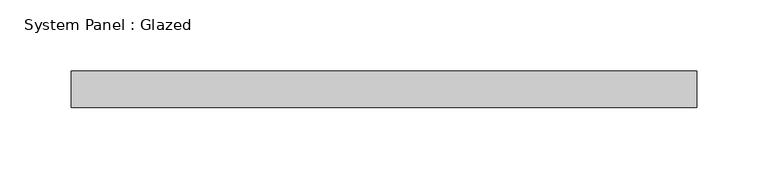
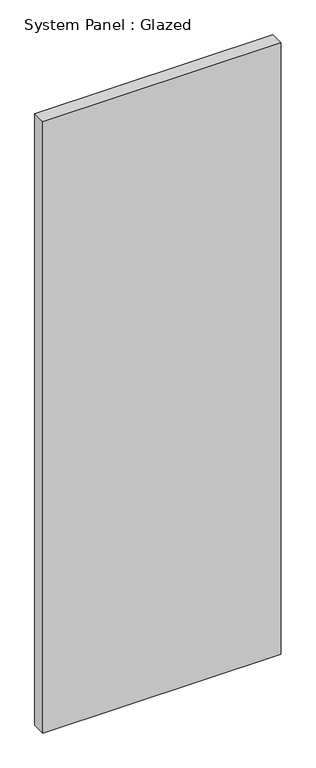
"""IFC4 building model written with IfcOpenShell, lengths in millimetres: plate geometry, System Panel : Glazed."""

from ifc_helpers import new_model, si_unit, origin, origin_with_axes, place, context, project, spatial, polyline, outline, extrude, source, transform, mapped, element, save


def system_panel_glazed_da88386f(model_context):
    return source(origin(), model_context, "Body", "SweptSolid", [
        extrude(outline(polyline([(219.075, 19.05), (-219.075, 19.05), (-219.075, 44.45), (219.075, 44.45), (219.075, 19.05)])), origin_with_axes(), (0.0, 0.0, 1.0), 1187.6685959),
    ])


if __name__ == "__main__":
    model = new_model("IFC4")
    model_context = context("Model", 3, world=origin())
    ifc_project = project(units=[si_unit("LENGTHUNIT", "METRE", prefix="MILLI")], contexts=[model_context])
    site = spatial("IfcSite", under=ifc_project)
    building = spatial("IfcBuilding", under=site)
    placement = place(None, origin())
    system_panel_glazed_shape = system_panel_glazed_da88386f(model_context)
    element("IfcPlate", 1, ObjectType="System Panel : Glazed", at=placement, inside=building, context=model_context, shape_type="MappedRepresentation", body=[
        mapped(system_panel_glazed_shape, transform((0.0, 0.0, 0.0), x_axis=(1.0, 0.0, 0.0), y_axis=(0.0, 1.0, 0.0), z_axis=(0.0, 0.0, 1.0))),
    ])
    save(model, "model.ifc")

# Revit data of these elements
# Type "System Panel : Glazed"
#   Construction Type Id = "GSP4R"
#   Analytic Construction = "1/8 in Pilkington single glazing"
#   Visual Light Transmittance = 0.9
#   Solar Heat Gain Coefficient = 0.86
#   Heat Transfer Coefficient (U) = 1.18115 BTU/(h·ft²·°F)
#   Define Thermal Properties by = 1
# Element 1 (IfcPlate, "System Panel : Glazed")
#   Materials on its faces: "Glass"
# Materials
#   "Glass": class "Glass", colour RGB 0 128 192, transparency 0.75, Description = "Soda Lime Glass", Cost = 0
